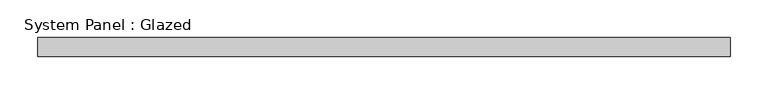
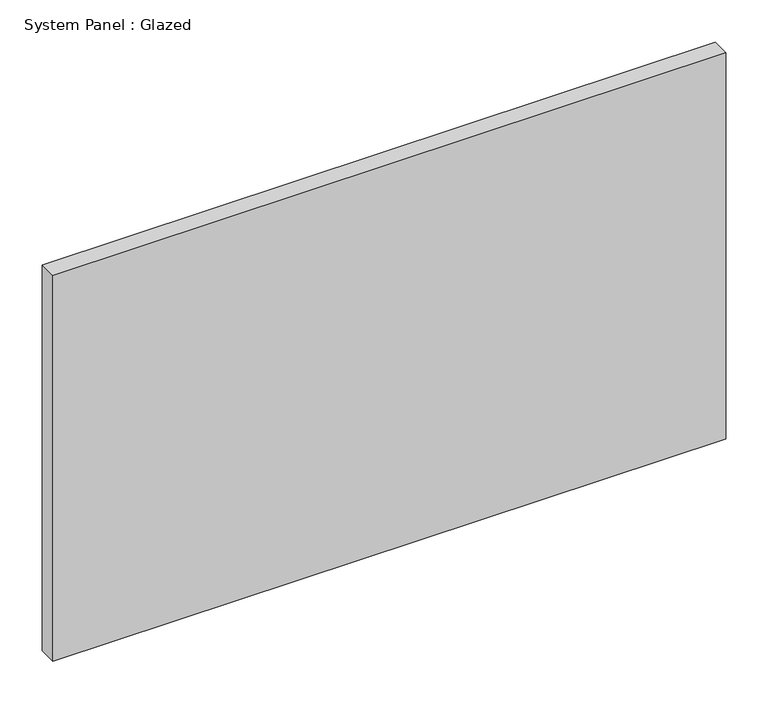
"""IFC4 building model written with IfcOpenShell, lengths in millimetres: plate geometry, System Panel : Glazed."""

from ifc_helpers import new_model, si_unit, origin, origin_with_axes, place, context, project, spatial, polyline, outline, extrude, source, transform, mapped, element, save


def system_panel_glazed_b16bc715(model_context):
    return source(origin(), model_context, "Body", "SweptSolid", [
        extrude(outline(polyline([(460.375, 19.05), (-460.375, 19.05), (-460.375, 44.45), (460.375, 44.45), (460.375, 19.05)])), origin_with_axes(), (0.0, 0.0, 1.0), 558.8),
    ])


if __name__ == "__main__":
    model = new_model("IFC4")
    model_context = context("Model", 3, world=origin())
    ifc_project = project(units=[si_unit("LENGTHUNIT", "METRE", prefix="MILLI")], contexts=[model_context])
    site = spatial("IfcSite", under=ifc_project)
    building = spatial("IfcBuilding", under=site)
    placement = place(None, origin())
    system_panel_glazed_shape = system_panel_glazed_b16bc715(model_context)
    element("IfcPlate", 1, ObjectType="System Panel : Glazed", at=placement, inside=building, context=model_context, shape_type="MappedRepresentation", body=[
        mapped(system_panel_glazed_shape, transform((0.0, 0.0, 0.0), x_axis=(1.0, 0.0, 0.0), y_axis=(0.0, 1.0, 0.0), z_axis=(0.0, 0.0, 1.0))),
    ])
    save(model, "model.ifc")

# Revit data of these elements
# Type "System Panel : Glazed"
#   Construction Type Id = "GSP4R"
#   Analytic Construction = "1/8 in Pilkington single glazing"
#   Visual Light Transmittance = 0.9
#   Solar Heat Gain Coefficient = 0.86
#   Heat Transfer Coefficient (U) = 1.18115 BTU/(h·ft²·°F)
#   Define Thermal Properties by = 1
# Element 1 (IfcPlate, "System Panel : Glazed")
#   Materials on its faces: "Glass"
# Materials
#   "Glass": class "Glass", colour RGB 0 128 192, transparency 0.75, Description = "Soda Lime Glass", Cost = 0
